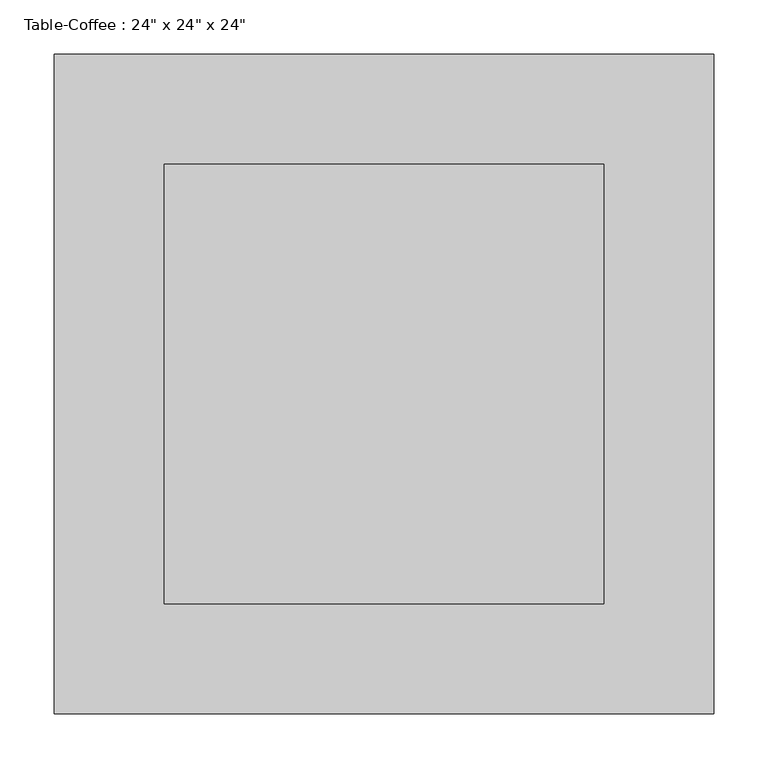
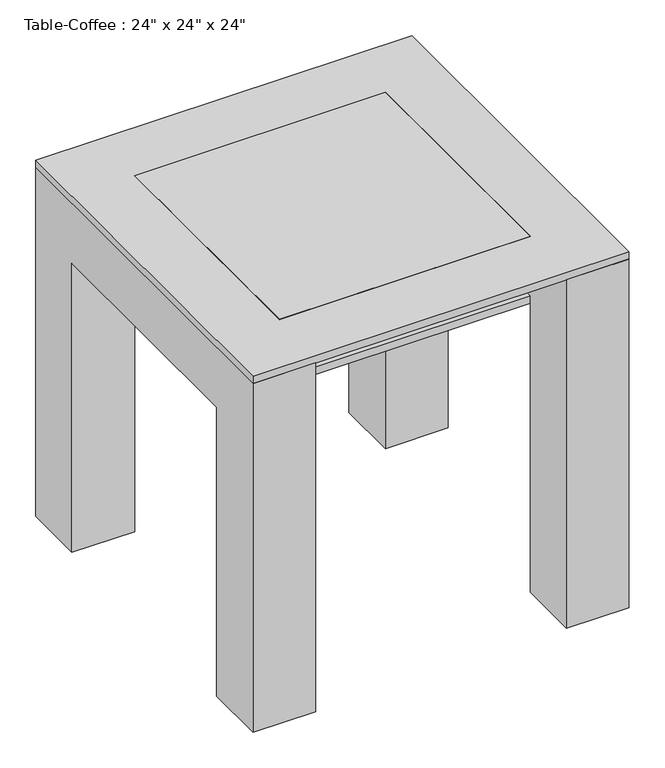
"""IFC4 building model written with IfcOpenShell, lengths in millimetres: furniture geometry."""

from ifc_helpers import new_model, si_unit, frame, origin, place, context, project, spatial, polyline, outline, extrude, source, transform, mapped, element, save


def furniture_b5c51a22(model_context):
    return source(origin(), model_context, "Body", "SweptSolid", [
        extrude(outline(polyline([(221.4657667, 298.4110778), (221.4657667, -107.9889222), (-184.9342333, -107.9889222), (-184.9342333, 298.4110778), (221.4657667, 298.4110778)])), frame((0.0, 0.0, 495.3), z_axis=(0.0, 0.0, 1.0), x_axis=(1.0, 0.0, 0.0)), (0.0, 0.0, 1.0), 12.7),
        extrude(outline(polyline([(400.0110778, 0.0), (298.4110778, 0.0), (298.4110778, 495.3), (-107.9889222, 495.3), (-107.9889222, 0.0), (-209.5889222, 0.0), (-209.5889222, 596.9), (400.0110778, 596.9), (400.0110778, 0.0)])), frame((221.4657667, 0.0, 0.0), z_axis=(1.0, 0.0, 0.0), x_axis=(0.0, 1.0, 0.0)), (0.0, 0.0, 1.0), 101.6),
        extrude(outline(polyline([(400.0110778, 596.9), (400.0110778, 0.0), (298.4110778, 0.0), (298.4110778, 495.3), (-107.9889222, 495.3), (-107.9889222, 0.0), (-209.5889222, 0.0), (-209.5889222, 596.9), (400.0110778, 596.9)])), frame((-286.5342333, 0.0, 0.0), z_axis=(1.0, 0.0, 0.0), x_axis=(0.0, 1.0, 0.0)), (0.0, 0.0, 1.0), 101.6),
        extrude(outline(polyline([(221.4657667, 298.4110778), (221.4657667, -107.9889222), (-184.9342333, -107.9889222), (-184.9342333, 298.4110778), (221.4657667, 298.4110778)])), frame((0.0, 0.0, 596.9), z_axis=(0.0, 0.0, 1.0), x_axis=(1.0, 0.0, 0.0)), (0.0, 0.0, 1.0), 12.7),
        extrude(outline(polyline([(323.0657667, 400.0110778), (323.0657667, -209.5889222), (-286.5342333, -209.5889222), (-286.5342333, 400.0110778), (323.0657667, 400.0110778)]), holes=[polyline([(221.4657667, 298.4110778), (-184.9342333, 298.4110778), (-184.9342333, -107.9889222), (221.4657667, -107.9889222), (221.4657667, 298.4110778)])]), frame((0.0, 0.0, 596.9), z_axis=(0.0, 0.0, 1.0), x_axis=(1.0, 0.0, 0.0)), (0.0, 0.0, 1.0), 12.7),
    ])


if __name__ == "__main__":
    model = new_model("IFC4")
    model_context = context("Model", 3, world=origin())
    ifc_project = project(units=[si_unit("LENGTHUNIT", "METRE", prefix="MILLI")], contexts=[model_context])
    site = spatial("IfcSite", under=ifc_project)
    building = spatial("IfcBuilding", under=site)
    placement = place(None, origin())
    furniture_shape = furniture_b5c51a22(model_context)
    element("IfcFurniture", 1, ObjectType="Table-Coffee : 24\" x 24\" x 24\"", at=placement, inside=building, context=model_context, shape_type="MappedRepresentation", body=[
        mapped(furniture_shape, transform((0.0, 0.0, 0.0), x_axis=(1.0, 0.0, 0.0), y_axis=(0.0, 1.0, 0.0), z_axis=(0.0, 0.0, 1.0))),
    ])
    save(model, "model.ifc")

# Revit data of these elements
# Type "Table-Coffee : 24\" x 24\" x 24\""
#   Assembly Code = "E2020200"
#   Height = 2' - 0"
#   Length = 2' - 0"
#   Width = 2' - 0"
#   Top Material = Wood
#   Frame Material = none
#   Default Elevation = 0
# Element 1 (IfcFurniture, "Table-Coffee : 24\" x 24\" x 24\"")
#   Materials on its faces: "Wood", "Glass - Clear, Grey"
# Materials
#   "Wood": class "Wood", colour RGB 0 0 0, transparency 0, Description = "Generic wood", Cost = 0
#   "Glass - Clear, Grey": class "Glass", colour RGB 252 255 255, transparency 0.64
